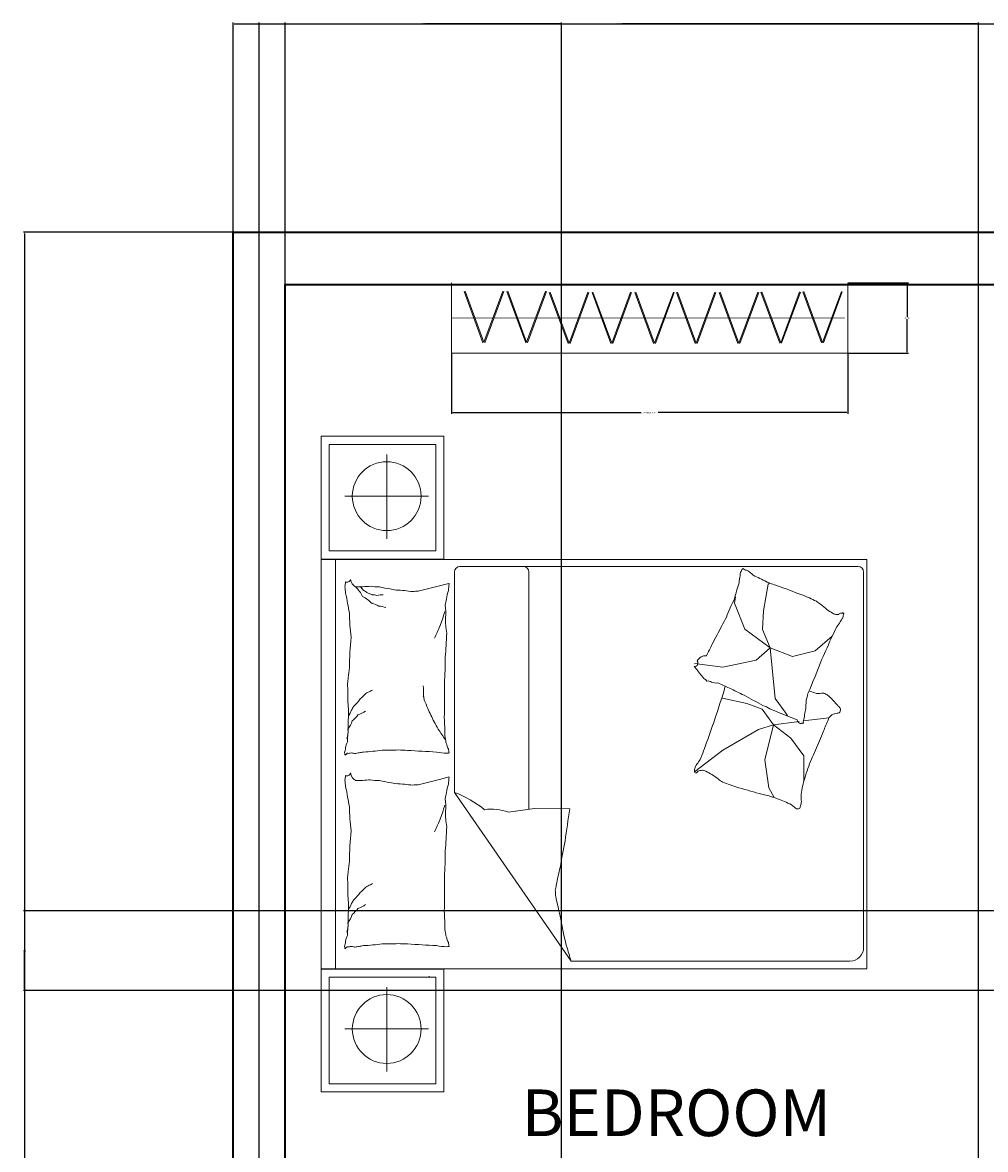
# Model space of a CAD drawing. Units: feet. Extents: x 1993 to 2298, y 2938 to 3641.
# Tile 9 of 11: x 1993 to 2141, y 3468 to 3641. Entities that reach past the tile are written whole.
import ezdxf

# ---------------------------------------------------------------- set-up
doc = ezdxf.new("R2010")
doc.units = ezdxf.units.FT
for name, color, linetype, lineweight in [('A-ANNO-DIMS', 2, 'Continuous', 18), ('A-AREA-IDEN', 7, 'Continuous', 18), ('furniture', 8, 'Continuous', 18), ('WAL', 7, 'Continuous', 35), ('wardrobe', 4, 'Continuous', 13)]:
    doc.layers.add(name, color=color, linetype=linetype, lineweight=lineweight)
doc.styles.add('DIM_FONT', font='SIMPLEX.shx', dxfattribs={"width": 0.8})
doc.styles.get("Standard").update_dxf_attribs({"font": 'arial.ttf'})
doc.dimstyles.get("Standard").update_dxf_attribs({"dimtxt": 0.18, "dimasz": 0.18, "dimexe": 0.18, "dimexo": 0.0625, "dimgap": 0.09, "dimtad": 0, "dimtih": 1, "dimtoh": 1, "dimdec": 4, "dimzin": 0, "dimdsep": 46, "dimtxsty": 'Standard', "dimcen": 0.09, "dimadec": 0, "dimazin": 0, "dimtfac": 1, "dimtdec": 4, "dimtofl": 0, "dimtmove": 0, "dimatfit": 3, "dimfxl": 1, "dimtolj": 1, "dimtzin": 0, "dimarcsym": 0})

# ---------------------------------------------------------------- blocks, each defined once
blk = doc.blocks.new('A$C79766A75')
for p, q in [((0.45, 1.9999), (0, 1.9999)), ((0, 1.9999), (0, 1.5499)), ((0.45, 1.5499), (0.45, 1.9999)), ((1.9506, 2), (0.4506, 2)), ((0.4506, 2), (0.4506, 0)), ((1.9506, 0), (1.9506, 2)), ((2.402, 1.9999), (1.952, 1.9999)), ((1.952, 1.9999), (1.952, 1.5499)), ((2.402, 1.5499), (2.402, 1.9999)), ((0.42, 1.9699), (0.03, 1.9699)), ((0.03, 1.9699), (0.03, 1.5799)), ((0.42, 1.5799), (0.42, 1.9699)), ((1.9506, 1.9476), (0.4506, 1.9476)), ((2.372, 1.9699), (1.982, 1.9699)), ((1.982, 1.9699), (1.982, 1.5799)), ((2.372, 1.5799), (2.372, 1.9699)), ((0.2304, 1.9125), (0.2304, 1.6061)), ((2.1824, 1.9125), (2.1824, 1.6061)), ((0.0743, 1.7595), (0.3834, 1.7595)), ((2.0263, 1.7595), (2.3354, 1.7595)), ((1.1461, 1.5617), (1.1254, 1.6443)), ((1.8553, 1.5617), (1.8346, 1.6443)), ((0.03, 1.5799), (0.42, 1.5799)), ((0.4234, 1.6034), (0.4228, 1.6034)), ((1.982, 1.5799), (2.372, 1.5799)), ((0, 1.5499), (0.45, 1.5499)), ((1.1536, 1.5317), (1.1461, 1.5617)), ((1.8628, 1.5317), (1.8553, 1.5617)), ((1.952, 1.5499), (2.402, 1.5499)), ((1.0972, 1.5115), (0.4791, 1.0841)), ((1.0972, 1.5115), (1.9048, 1.5115)), ((1.9248, 1.4915), (1.9248, 0.0322)), ((1.0383, 1.2184), (1.0246, 1.3138)), ((1.9048, 1.2389), (1.0354, 1.2389)), ((1.0365, 1.0883), (1.0383, 1.2184)), ((0.4791, 0.0622), (0.4791, 1.0841)), ((1.1731, 0.6316), (1.2523, 0.5276)), ((1.5696, 0.6317), (1.5559, 0.5286)), ((1.2523, 0.5276), (1.3274, 0.3973)), ((1.4223, 0.4407), (1.442, 0.5296)), ((1.5559, 0.5286), (1.5817, 0.4065)), ((1.6952, 0.4478), (1.7898, 0.4856)), ((1.7898, 0.4856), (1.8139, 0.4822)), ((1.4025, 0.3834), (1.4223, 0.4407)), ((1.6264, 0.355), (1.6952, 0.4478)), ((1.2167, 0.3736), (1.1139, 0.3597)), ((1.3452, 0.342), (1.2167, 0.3736)), ((1.3274, 0.3973), (1.3452, 0.342)), ((1.3452, 0.342), (1.4025, 0.3834)), ((1.5817, 0.4065), (1.6264, 0.355)), ((1.6264, 0.355), (1.6935, 0.3825)), ((1.6935, 0.3825), (1.7623, 0.379)), ((1.7623, 0.379), (1.8603, 0.3619)), ((1.1139, 0.3597), (1.0779, 0.3397)), ((1.2957, 0.2787), (1.3452, 0.342)), ((1.3452, 0.342), (1.3569, 0.2478)), ((1.4034, 0.3558), (1.3803, 0.2995)), ((1.4406, 0.3361), (1.3907, 0.3)), ((1.6264, 0.355), (1.4406, 0.3361)), ((1.5954, 0.2725), (1.6264, 0.355)), ((1.8603, 0.3619), (1.8636, 0.3554)), ((1.3803, 0.2995), (1.3626, 0.256)), ((1.3907, 0.3), (1.3787, 0.2914)), ((1.2305, 0.2313), (1.2957, 0.2787)), ((1.6161, 0.19), (1.5954, 0.2725)), ((1.1376, 0.2313), (1.2305, 0.2313)), ((1.3588, 0.2331), (1.3706, 0.1385)), ((1.6697, 0.1274), (1.6161, 0.19)), ((1.9048, 0.0122), (0.5291, 0.0122)), ((0.4506, 0), (1.9506, 0))]:
    blk.add_line(p, q)
for centre in [(0.2304, 1.7595), (2.1824, 1.7595)]:
    blk.add_circle(centre, 0.126)
for centre, radius, start, end in [((0.5232, 1.9139), 0.00342, 291.7883, 340.436), ((0.525, 1.9085), 0.00232, 340.436, 101.8931), ((0.5246, 1.9378), 0.0251, 274.3025, 291.7883), ((0.5311, 1.9093), 0.00428, 201.9904, 281.8931), ((0.5465, 1.8994), 0.0156, 158.579, 201.9904), ((0.5486, 1.9393), 0.0289, 239.3487, 274.3025), ((0.5458, 1.8568), 0.0539, 59.3487, 84.7408), ((0.546, 1.0829), 0.8208, 84.7408, 88.0921), ((0.6118, 2.0005), 0.0992, 254.0648, 274.2159), ((0.6775, 1.9817), 0.0992, 233.9136, 254.0648), ((0.6362, 0.406), 1.4943, 88.0921, 90.5757), ((0.7737, 2.1075), 0.234, 242.7604, 249.1397), ((0.7591, 1.0293), 0.8732, 90.5757, 94.8018), ((0.7631, 2.1919), 0.2897, 267.4614, 274.8018), ((0.8143, 2.0532), 0.1524, 259.8101, 267.4614), ((0.7515, 1.3747), 0.5293, 79.8101, 83.9133), ((1.1117, 1.6625), 0.2422, 97.5469, 105.744), ((1.0352, 2.2041), 0.3048, 278.4372, 285.744), ((1.1179, 2.0719), 0.1611, 270, 278.4372), ((1.1592, 2.0011), 0.0904, 258.7276, 270), ((1.1709, 1.9049), 0.0131, 153.4195, 258.7276), ((1.2325, 1.9139), 0.00342, 291.7883, 340.436), ((1.2342, 1.9085), 0.00232, 340.436, 101.8931), ((1.2338, 1.9378), 0.0251, 274.3025, 291.7883), ((1.2404, 1.9093), 0.00428, 201.9904, 281.8931), ((1.2558, 1.8994), 0.0156, 158.579, 201.9904), ((1.2578, 1.9393), 0.0289, 239.3487, 274.3025), ((1.2551, 1.8568), 0.0539, 59.3487, 84.7408), ((1.2552, 1.0829), 0.8208, 84.7408, 88.0921), ((1.3211, 2.0005), 0.0992, 254.0648, 274.2159), ((1.3868, 1.9817), 0.0992, 233.9136, 254.0648), ((1.3455, 0.406), 1.4943, 88.0921, 90.5757), ((1.4829, 2.1075), 0.234, 242.7604, 249.1397), ((1.4683, 1.0293), 0.8732, 90.5757, 94.8018), ((1.4724, 2.1919), 0.2897, 267.4614, 274.8018), ((1.5236, 2.0532), 0.1524, 259.8101, 267.4614), ((1.4607, 1.3747), 0.5293, 79.8101, 83.9133), ((1.821, 1.6625), 0.2422, 97.5469, 105.744), ((1.7444, 2.2041), 0.3048, 278.4372, 285.744), ((1.8271, 2.0719), 0.1611, 270, 278.4372), ((1.8684, 2.0011), 0.0904, 258.7276, 270), ((1.8802, 1.9049), 0.0131, 153.4195, 258.7276), ((0.4996, 1.8889), 0.0328, 338.579, 8.1335), ((0.2896, 1.8253), 0.246, 8.1335, 12.1095), ((0.7297, 1.8867), 0.1983, 187.6809, 192.1095), ((0.7304, 1.9449), 0.0992, 216.1766, 233.9136), ((0.7661, 1.8961), 0.0992, 198.4397, 216.1766), ((0.738, 1.949), 0.0768, 231.6114, 242.7604), ((0.974, 2.1633), 0.3916, 226.1885, 231.6114), ((0.8451, 0.8466), 1.049, 83.9133, 90), ((1.046, 1.2129), 0.6827, 90, 97.5469), ((1.171, 1.8579), 0.0342, 94.4002, 153.4195), ((1.6324, 1.8735), 0.4918, 180, 186.2324), ((1.2088, 1.8889), 0.0328, 338.579, 8.1335), ((0.9988, 1.8253), 0.246, 8.1335, 12.1095), ((1.4389, 1.8867), 0.1983, 187.6809, 192.1095), ((1.4396, 1.9449), 0.0992, 216.1766, 233.9136), ((1.4753, 1.8961), 0.0992, 198.4397, 216.1766), ((1.4473, 1.949), 0.0768, 231.6114, 242.7604), ((1.6833, 2.1633), 0.3916, 226.1885, 231.6114), ((1.5543, 0.8466), 1.049, 83.9133, 90), ((1.7552, 1.2129), 0.6827, 90, 97.5469), ((1.7511, 1.9723), 0.1399, 297.2036, 314.9024), ((1.8802, 1.8579), 0.0342, 94.4002, 153.4195), ((2.3416, 1.8735), 0.4918, 180, 186.2324), ((1.4472, 1.8987), 0.9131, 183.3687, 187.6809), ((0.9057, 1.9982), 0.2252, 219.0349, 226.1885), ((0.7932, 1.8591), 0.0493, 208.3168, 219.0349), ((0.9392, 1.9062), 0.2002, 203.0028, 208.3168), ((1.3446, 1.7858), 0.204, 170.3156, 180), ((2.1565, 1.8987), 0.9131, 183.3687, 187.6809), ((1.615, 1.9982), 0.2252, 219.0349, 226.1885), ((1.5025, 1.8591), 0.0493, 208.3168, 219.0349), ((1.6484, 1.9062), 0.2002, 203.0028, 208.3168), ((1.6908, 1.9123), 0.1399, 314.9024, 332.6012), ((1.6307, 1.8895), 0.2056, 338.1851, 341.2201), ((1.6887, 1.8881), 0.1511, 334.6449, 338.1851), ((1.7896, 1.8667), 0.0526, 318.5571, 334.6449), ((1.784, 1.9167), 0.0899, 306.2641, 318.5571), ((2.0538, 1.7858), 0.204, 170.3156, 180), ((1.2208, 1.7573), 0.6787, 178.3669, 183.3687), ((2.0027, 1.5994), 0.882, 167.8016, 170.3156), ((1.9301, 1.7573), 0.6787, 178.3669, 183.3687), ((1.6404, 1.8023), 0.1399, 343.485, 354.3689), ((1.6554, 1.8529), 0.1399, 332.6012, 343.485), ((1.7653, 1.8132), 0.0562, 341.2201, 0), ((1.73, 1.7719), 0.0915, 0, 14.6851), ((2.7119, 1.5994), 0.882, 167.8016, 170.3156), ((0.8192, 1.792), 0.3171, 347.8016, 351.9949), ((1.5284, 1.792), 0.3171, 347.8016, 351.9949), ((1.9066, 1.6447), 1.3652, 176.945, 178.3669), ((0.4711, 1.7556), 0.6588, 351.9949, 357.3351), ((2.6158, 1.6447), 1.3652, 176.945, 178.3669), ((1.1803, 1.7556), 0.6588, 351.9949, 357.3351), ((14.1519, 0.85), 13.6356, 176.49514, 176.94504), ((1.0578, 1.6474), 0.0677, 357.3351, 14.0452), ((14.8612, 0.85), 13.6356, 176.49514, 176.94504), ((1.767, 1.6474), 0.0677, 357.3351, 14.0452), ((1.226, 2.0834), 0.5066, 290.6743, 294.3265), ((1.4305, 1.6796), 0.058, 274.0828, 290.6743), ((1.4679, 1.8969), 0.2721, 266.4448, 274.0828), ((0.8521, 1.5209), 0.3212, 170.0016, 176.4951), ((0.6583, 0.9067), 0.7387, 64.6889, 66.5156), ((0.7015, 0.888), 0.7387, 66.5156, 68.3423), ((1.5613, 1.5209), 0.3212, 170.0016, 176.4951), ((0.9025, 2.1618), 0.7286, 302.135, 305.8263), ((1.1895, 1.8508), 0.3126, 296.4985, 302.135), ((0.7658, 2.8912), 1.4323, 294.3265, 296.4985), ((1.3675, 0.9067), 0.7387, 64.6889, 66.5156), ((1.4107, 0.888), 0.7387, 66.5156, 68.3423), ((0.513, 1.535), 0.0193, 350.0016, 16.6978), ((0.5322, 1.5304), 0.00132, 16.6978, 97.1204), ((0.5579, 1.4467), 0.0875, 97.1204, 106.2212), ((0.5822, 1.4654), 0.0767, 106.2212, 117.2841), ((0.5507, 1.5832), 0.0453, 282.869, 297.2841), ((0.5623, 1.6885), 0.1459, 273.574, 282.869), ((0.589, 2.7103), 1.164, 270.2865, 273.574), ((0.7584, 7.2662), 5.7185, 269.0296, 270.2865), ((0.9401, 4.9065), 3.3622, 267.3904, 269.0296), ((0.9811, 2.7573), 1.2165, 265.3824, 267.3904), ((0.8583, 0.139), 1.4048, 85.3824, 87.2509), ((1.0175, 1.3138), 0.2301, 87.2509, 101.5586), ((0.7501, 0.8688), 0.7387, 68.3423, 70.572), ((0.8043, 0.8497), 0.7387, 70.572, 72.8018), ((1.0449, 1.6886), 0.1459, 263.5659, 281.5586), ((1.1099, 1.6599), 0.1197, 252.6136, 263.5659), ((1.0587, 1.3144), 0.2297, 72.6136, 80.5159), ((1.108, 1.2635), 0.2708, 80.5159, 85.9171), ((1.1535, 1.5308), 0.000917, 85.9171, 194.0449), ((1.2222, 1.535), 0.0193, 350.0016, 16.6978), ((1.2414, 1.5304), 0.00132, 16.6978, 97.1204), ((1.2671, 1.4467), 0.0875, 97.1204, 106.2212), ((1.2914, 1.4654), 0.0767, 106.2212, 117.2841), ((1.2599, 1.5832), 0.0453, 282.869, 297.2841), ((1.2716, 1.6885), 0.1459, 273.574, 282.869), ((1.2982, 2.7103), 1.164, 270.2865, 273.574), ((1.4677, 7.2662), 5.7185, 269.0296, 270.2865), ((1.6493, 4.9065), 3.3622, 267.3904, 269.0296), ((1.6903, 2.7573), 1.2165, 265.3824, 267.3904), ((1.5676, 0.139), 1.4048, 85.3824, 87.2509), ((1.7268, 1.3138), 0.2301, 87.2509, 101.5586), ((1.4594, 0.8688), 0.7387, 68.3423, 70.572), ((1.5136, 0.8497), 0.7387, 70.572, 72.8018), ((1.7541, 1.6886), 0.1459, 263.5659, 281.5586), ((1.8192, 1.6599), 0.1197, 252.6136, 263.5659), ((1.7679, 1.3144), 0.2297, 72.6136, 80.5159), ((1.8172, 1.2635), 0.2708, 80.5159, 85.9171), ((1.8627, 1.5308), 0.000917, 85.9171, 194.0449), ((0.745, 1.6407), 0.3751, 320.3555, 339.8512), ((1.9048, 1.4915), 0.02, 0, 90), ((0.8556, 1.3759), 0.1801, 339.8512, 8.1356), ((1.9048, 1.2589), 0.02, 270, 0), ((-0.1888, 5.1029), 4.0646, 280.7276, 282.9255), ((0.7282, 1.1989), 0.0581, 262.2696, 280.7276), ((0.7833, 1.3309), 0.1942, 256.8096, 262.2696), ((0.2481, -1.3253), 2.5158, 76.8096, 78.3259), ((0.3953, -1.4284), 2.588, 78.3259, 80.505), ((-0.0248, 2.8487), 1.8351, 285.9352, 287.7364), ((0.3872, 1.7415), 0.6574, 282.9255, 285.9352), ((0.413, -2.64), 3.7801, 80.505, 82.308), ((1.1752, 0.6267), 0.0063, 166.7192, 233.4208), ((1.1734, 0.6272), 0.00443, 93.9484, 166.7192), ((1.163, 0.6103), 0.0142, 10.4074, 53.4208), ((1.1755, 0.5964), 0.0352, 69.6548, 93.9484), ((1.1669, 0.5731), 0.0601, 51.4146, 69.6548), ((1.2538, 0.682), 0.0792, 231.4146, 247.2931), ((1.1426, 1.1456), 0.6605, 306.2163, 307.2151), ((1.7751, 0.3162), 0.3825, 126.2163, 127.5287), ((1.5806, 0.5924), 0.0452, 127.5287, 134.1274), ((1.5093, 0.6825), 0.0697, 308.8136, 314.1274), ((1.5706, 0.6318), 0.0127, 176.7545, 308.8136), ((1.5621, 0.59), 0.0359, 356.7545, 62.7098), ((0.8605, 0.749), 0.352, 329.0944, 333.1821), ((1.1396, 0.6079), 0.0393, 333.1821, 345.4291), ((1.1011, 0.5989), 0.0771, 2.7286, 10.4074), ((1.1628, 0.6019), 0.0153, 345.4291, 2.7286), ((1.5463, 1.3811), 0.8371, 247.2931, 249.8713), ((3.0113, 5.3783), 5.0942, 249.8713, 250.9164), ((1.4828, 0.5833), 0.0226, 324.1064, 8.0492), ((1.4519, 0.6426), 0.0774, 313.5224, 324.1064), ((1.383, 0.7705), 0.2176, 307.2151, 313.5224), ((0.2201, -2.1858), 3.0972, 62.7098, 63.5853), ((1.2077, 0.4922), 0.081, 140.2995, 153.9265), ((0.9961, 0.6678), 0.194, 320.2995, 329.0944), ((2.374, 3.5362), 3.145, 250.9164, 253.3915), ((2.4089, 0.1204), 1.0054, 154.9471, 157.5838), ((1.5435, 0.5526), 0.0458, 157.5838, 188.0492), ((2.5711, 2.3551), 2.0162, 242.5001, 243.5853), ((4.5245, 5.9445), 6.1019, 242.15178, 242.50014), ((3.0311, -0.112), 2.003, 162.1604, 164.7375), ((1.3115, 0.4414), 0.1965, 153.9265, 162.1604), ((2.9813, -0.2643), 1.6868, 152.9116, 154.9471), ((1.5084, 0.6341), 0.1166, 253.3915, 259.2634), ((-0.9881, -4.647), 5.8383, 62.15178, 62.50792), ((1.5182, -0.068), 0.6236, 62.5079, 69.2514), ((1.7121, 0.0657), 0.43, 69.2514, 77.3748), ((1.8682, 0.4049), 0.063, 77.3748, 93.3881), ((1.8955, 0.5247), 0.0599, 256.9598, 273.3881), ((1.9257, 0.5082), 0.0509, 238.3083, 256.9598), ((1.9201, 0.4587), 0.0058, 180.9614, 238.3083), ((2.6887, -0.0186), 1.6481, 164.7375, 166.159), ((2.8096, -0.3311), 1.5652, 150.064, 152.9116), ((-0.5166, 1.5491), 2.6619, 333.6668, 334.8268), ((1.8435, 0.4743), 0.0755, 310.5086, 333.6668), ((1.9279, 0.441), 0.0168, 130.5086, 180.9614), ((0.5589, 0.5062), 0.5454, 343.6878, 346.159), ((1.2176, 0.4627), 0.2143, 330.064, 337.7645), ((-1.4109, 1.284), 2.6619, 338.0627, 339.2227), ((0.9098, 0.4035), 0.1798, 339.2227, 343.6878), ((3.4079, -0.2212), 1.6481, 160.3416, 161.7631), ((1.3456, 0.5261), 0.5454, 339.2919, 341.7631), ((1.701, 0.4319), 0.1798, 334.8268, 339.2919), ((0.9882, 0.3177), 0.0755, 314.9045, 338.0627), ((3.6966, -0.4634), 2.003, 157.7645, 160.3416), ((1.0533, 0.2524), 0.0168, 134.9045, 185.3572), ((1.0424, 0.2513), 0.0058, 185.3572, 242.7041), ((1.3694, 0.234), 0.0231, 107.1867, 157.7645), ((1.0631, 0.2914), 0.0509, 242.7041, 261.3557), ((1.0645, 0.3003), 0.0599, 261.3557, 277.784), ((1.0811, 0.1786), 0.063, 81.7707, 97.784), ((1.0286, -0.1846), 0.43, 73.6473, 81.7707), ((0.974, -0.3705), 0.6236, 66.9038, 73.6473), ((1.3465, 0.2383), 0.00467, 287.1867, 70.6201), ((1.3486, 0.2247), 0.0092, 70.6201, 94.2593), ((1.3563, 0.267), 0.034, 262.0178, 274.2593), ((1.4091, 0.4221), 0.1955, 255.1193, 262.0178), ((1.358, 0.0507), 0.1794, 75.1193, 82.3216), ((1.4096, 0.153), 0.0712, 82.3216, 94.5118), ((1.4285, 0.2893), 0.0663, 261.8784, 274.5118), ((1.4755, 0.332), 0.1166, 248.9957, 261.8784), ((2.7121, 3.1012), 3.145, 246.5205, 248.9957), ((2.4175, -0.1202), 1.0054, 160.6552, 161.9797), ((1.9797, 0.1108), 0.1965, 149.5306, 157.7645), ((-1.0716, -5.1672), 5.8383, 66.54766, 66.9038), ((3.6805, 5.7866), 6.1019, 246.54766, 246.89602), ((2.0773, 2.0287), 2.0162, 246.896, 247.9812), ((1.4382, 0.1619), 0.0226, 328.5023, 12.4451), ((1.505, 0.1766), 0.0458, 161.9797, 192.4451), ((3.6993, 4.7998), 5.0942, 245.4754, 246.5205), ((1.6279, 0.2819), 0.194, 315.9036, 324.6985), ((1.856, 0.1288), 0.081, 135.9036, 149.5306), ((0.1602, -2.7118), 3.0972, 67.1056, 67.9812), ((1.3512, 0.1084), 0.0359, 1.1504, 67.1056), ((1.2874, 0.2845), 0.2176, 311.611, 317.9183), ((1.3914, 0.1905), 0.0774, 317.9183, 328.5023), ((2.051, 0.8725), 0.8371, 242.8972, 245.4754), ((1.7162, 0.1388), 0.0393, 328.7862, 341.0332), ((1.4661, 0.3294), 0.352, 324.6985, 328.7862), ((1.3997, 0.1094), 0.0127, 181.1504, 313.2095), ((1.3607, 0.1509), 0.0697, 313.2095, 318.5233), ((1.4468, 0.0748), 0.0452, 131.9246, 138.5233), ((1.6722, -0.1762), 0.3825, 130.6122, 131.9246), ((0.9933, 0.6156), 0.6605, 310.6122, 311.611), ((1.7576, 0.1689), 0.0792, 227.0187, 242.8972), ((1.6963, 0.0438), 0.0601, 47.0187, 65.2589), ((1.737, 0.0526), 0.0352, 65.2589, 89.5525), ((1.7345, 0.1188), 0.0153, 341.0332, 358.3327), ((1.6723, 0.1058), 0.0771, 358.3327, 6.0115), ((1.7401, 0.0928), 0.0142, 6.0115, 49.0249), ((1.756, 0.0832), 0.00443, 89.5525, 162.3233), ((1.7602, 0.0924), 0.0063, 162.3233, 229.0249), ((0.5291, 0.0622), 0.05, 180, 270), ((1.9048, 0.0322), 0.02, 270, 0)]:
    blk.add_arc(centre, radius, start, end)
at = {"style": 'DIM_FONT', "text_generation_flag": 4, "width": 0.8, "flags": 9}
for tag in ['XSIZE', 'YSIZE']:
    blk.add_attdef(tag, (1.9506, 2), '', height=0.0005, rotation=180, dxfattribs=at)
blk = doc.blocks.new('WARDROBE-PLAN')
for p, q in [((4.82, 1.61), (1.93, 9.47)), ((4.96, 1.67), (2.08, 9.52)), ((4.96, 1.67), (7.85, 9.52)), ((5.11, 1.61), (7.99, 9.46)), ((11.37, 1.61), (8.49, 9.46)), ((11.51, 1.67), (8.63, 9.52)), ((11.51, 1.67), (14.4, 9.52)), ((11.66, 1.61), (14.54, 9.46)), ((17.87, 1.47), (14.98, 9.32)), ((18.01, 1.52), (15.13, 9.37)), ((18.01, 1.52), (20.9, 9.37)), ((18.16, 1.47), (21.04, 9.32)), ((24.42, 1.47), (21.53, 9.32)), ((24.56, 1.52), (21.68, 9.37)), ((24.56, 1.52), (27.45, 9.37)), ((24.71, 1.47), (27.59, 9.32)), ((30.97, 1.47), (28.09, 9.32)), ((31.11, 1.52), (28.23, 9.37)), ((31.11, 1.52), (34, 9.37)), ((31.26, 1.47), (34.14, 9.32)), ((37.35, 1.47), (34.47, 9.32)), ((37.5, 1.52), (34.62, 9.37)), ((37.5, 1.52), (40.38, 9.37)), ((37.64, 1.47), (40.53, 9.32)), ((43.9, 1.46), (41.02, 9.32)), ((44.05, 1.52), (41.17, 9.37)), ((44.05, 1.52), (46.93, 9.37)), ((44.19, 1.46), (47.08, 9.32)), ((50.31, 1.52), (47.43, 9.37)), ((50.46, 1.57), (47.57, 9.42)), ((50.46, 1.57), (53.34, 9.42)), ((50.6, 1.52), (53.49, 9.37)), ((56.72, 1.57), (53.83, 9.42)), ((56.86, 1.62), (53.98, 9.47)), ((56.86, 1.62), (59.75, 9.47)), ((57.01, 1.57), (59.89, 9.42)), ((0, 5.4), (60.23, 5.39))]:
    blk.add_line(p, q)
blk.add_lwpolyline([(0, 10.78), (0, 0.01), (60.75, 0), (60.75, 10.78)])
blk = doc.blocks.new('*D36')
at = {"layer": 'A-ANNO-DIMS', "color": 0, "lineweight": -2, "transparency": 16777216}
for p, q in [((2059.25, 3589.94), (2059.25, 3580.71)), ((2120, 3589.94), (2120, 3580.71)), ((2059.43, 3580.89), (2088.32, 3580.89)), ((2119.82, 3580.89), (2090.93, 3580.89))]:
    blk.add_line(p, q, dxfattribs=at)
at = {"layer": 'A-ANNO-DIMS', "color": 0, "transparency": 16777216}
for points in [[(2059.43, 3580.92), (2059.43, 3580.86), (2059.25, 3580.89)], [(2119.82, 3580.92), (2119.82, 3580.86), (2120, 3580.89)]]:
    blk.add_solid(points, dxfattribs=at)
at = {"layer": 'Defpoints', "color": 0, "transparency": 16777216}
for p in [(2059.25, 3590), (2120, 3590), (2120, 3580.89)]:
    blk.add_point(p, dxfattribs=at)
at = {"layer": 'A-ANNO-DIMS', "color": 0, "transparency": 16777216, "insert": (2089.62, 3580.89), "char_height": 0.18, "attachment_point": 5}
blk.add_mtext('\\A1;WARDROBE 61 TYP.', dxfattribs=at)
blk = doc.blocks.new('*D37')
at = {"layer": 'A-ANNO-DIMS', "color": 0, "lineweight": -2, "transparency": 16777216}
for p, q in [((2120.06, 3600.78), (2129.29, 3600.78)), ((2129.11, 3600.6), (2129.11, 3595.57)), ((2129.11, 3590.18), (2129.11, 3595.21)), ((2120.06, 3590), (2129.29, 3590))]:
    blk.add_line(p, q, dxfattribs=at)
at = {"layer": 'A-ANNO-DIMS', "color": 0, "transparency": 16777216}
for points in [[(2129.08, 3600.6), (2129.14, 3600.6), (2129.11, 3600.78)], [(2129.08, 3590.18), (2129.14, 3590.18), (2129.11, 3590)]]:
    blk.add_solid(points, dxfattribs=at)
at = {"layer": 'Defpoints', "color": 0, "transparency": 16777216}
for p in [(2120, 3600.78), (2129.11, 3600.78), (2120, 3590)]:
    blk.add_point(p, dxfattribs=at)
at = {"layer": 'A-ANNO-DIMS', "color": 0, "transparency": 16777216, "insert": (2129.11, 3595.39), "char_height": 0.18, "attachment_point": 5}
blk.add_mtext('\\A1;11 TYP.', dxfattribs=at)
blk = doc.blocks.new('*D54')
at = {"layer": 'A-ANNO-DIMS', "color": 0, "lineweight": -2, "transparency": 16777216}
for p, q in [((2025.76, 3608.6), (2025.76, 3640.68)), ((2025.94, 3640.5), (2145.47, 3640.5)), ((2265.58, 3640.5), (2146.05, 3640.5)), ((2265.76, 3608.6), (2265.76, 3640.68))]:
    blk.add_line(p, q, dxfattribs=at)
at = {"layer": 'A-ANNO-DIMS', "color": 0, "transparency": 16777216}
for points in [[(2025.94, 3640.53), (2025.94, 3640.47), (2025.76, 3640.5)], [(2265.58, 3640.53), (2265.58, 3640.47), (2265.76, 3640.5)]]:
    blk.add_solid(points, dxfattribs=at)
at = {"layer": 'Defpoints', "color": 0, "transparency": 16777216}
for p in [(2265.76, 3640.5), (2025.76, 3608.53), (2265.76, 3608.53)]:
    blk.add_point(p, dxfattribs=at)
at = {"layer": 'A-ANNO-DIMS', "color": 0, "transparency": 16777216, "insert": (2145.76, 3640.5), "char_height": 0.18, "attachment_point": 5}
blk.add_mtext('\\A1;240', dxfattribs=at)
blk = doc.blocks.new('*D56')
at = {"layer": 'A-ANNO-DIMS', "color": 0, "lineweight": -2, "transparency": 16777216}
for p, q in [((2025.7, 3608.53), (1993.61, 3608.53)), ((1993.79, 3608.35), (1993.79, 3289.45)), ((1993.79, 2970.18), (1993.79, 3289.08)), ((2029.7, 2970), (1993.61, 2970))]:
    blk.add_line(p, q, dxfattribs=at)
at = {"layer": 'A-ANNO-DIMS', "color": 0, "transparency": 16777216}
for points in [[(1993.76, 3608.35), (1993.82, 3608.35), (1993.79, 3608.53)], [(1993.76, 2970.18), (1993.82, 2970.18), (1993.79, 2970)]]:
    blk.add_solid(points, dxfattribs=at)
at = {"layer": 'Defpoints', "color": 0, "transparency": 16777216}
for p in [(1993.79, 3608.53), (2025.76, 3608.53), (2029.76, 2970)]:
    blk.add_point(p, dxfattribs=at)
at = {"layer": 'A-ANNO-DIMS', "color": 0, "transparency": 16777216, "insert": (1993.79, 3289.27), "char_height": 0.18, "attachment_point": 5}
blk.add_mtext('\\A1;638.5', dxfattribs=at)
blk = doc.blocks.new('*D59')
at = {"layer": 'A-ANNO-DIMS', "color": 0, "lineweight": -2, "transparency": 16777216}
for p, q in [((2140, 3048.6), (2140, 3640.68)), ((2140.18, 3640.5), (2144.79, 3640.5)), ((2149.82, 3640.5), (2145.21, 3640.5)), ((2150, 3048.6), (2150, 3640.68))]:
    blk.add_line(p, q, dxfattribs=at)
at = {"layer": 'A-ANNO-DIMS', "color": 0, "transparency": 16777216}
for points in [[(2140.18, 3640.53), (2140.18, 3640.47), (2140, 3640.5)], [(2149.82, 3640.53), (2149.82, 3640.47), (2150, 3640.5)]]:
    blk.add_solid(points, dxfattribs=at)
at = {"layer": 'Defpoints', "color": 0, "transparency": 16777216}
for p in [(2150, 3640.5), (2140, 3048.53), (2150, 3048.53)]:
    blk.add_point(p, dxfattribs=at)
at = {"layer": 'A-ANNO-DIMS', "color": 0, "transparency": 16777216, "insert": (2145, 3640.5), "char_height": 0.18, "attachment_point": 5}
blk.add_mtext('\\A1;10', dxfattribs=at)
blk = doc.blocks.new('*D70')
at = {"layer": 'A-ANNO-DIMS', "color": 0, "lineweight": -2, "transparency": 16777216}
for p, q in [((2149.7, 3504.53), (1993.61, 3504.53)), ((1993.79, 3504.35), (1993.79, 3498.61)), ((1993.79, 3492.51), (1993.79, 3498.25)), ((2149.7, 3492.33), (1993.61, 3492.33))]:
    blk.add_line(p, q, dxfattribs=at)
at = {"layer": 'A-ANNO-DIMS', "color": 0, "transparency": 16777216}
for points in [[(1993.76, 3504.35), (1993.82, 3504.35), (1993.79, 3504.53)], [(1993.76, 3492.51), (1993.82, 3492.51), (1993.79, 3492.33)]]:
    blk.add_solid(points, dxfattribs=at)
at = {"layer": 'Defpoints', "color": 0, "transparency": 16777216}
for p in [(1993.79, 3504.53), (2149.76, 3504.53), (2149.76, 3492.33)]:
    blk.add_point(p, dxfattribs=at)
at = {"layer": 'A-ANNO-DIMS', "color": 0, "transparency": 16777216, "insert": (1993.79, 3498.43), "char_height": 0.18, "attachment_point": 5}
blk.add_mtext('\\A1;12.2', dxfattribs=at)
blk = doc.blocks.new('*D75')
at = {"layer": 'A-ANNO-DIMS', "color": 0, "lineweight": -2, "transparency": 16777216}
for p, q in [((2029.76, 3008.6), (2029.76, 3640.68)), ((2029.94, 3640.5), (2084.42, 3640.5)), ((2139.82, 3640.5), (2085.33, 3640.5)), ((2140, 3008.6), (2140, 3640.68))]:
    blk.add_line(p, q, dxfattribs=at)
at = {"layer": 'A-ANNO-DIMS', "color": 0, "transparency": 16777216}
for points in [[(2029.94, 3640.53), (2029.94, 3640.47), (2029.76, 3640.5)], [(2139.82, 3640.53), (2139.82, 3640.47), (2140, 3640.5)]]:
    blk.add_solid(points, dxfattribs=at)
at = {"layer": 'Defpoints', "color": 0, "transparency": 16777216}
for p in [(2140, 3640.5), (2029.76, 3008.53), (2140, 3008.53)]:
    blk.add_point(p, dxfattribs=at)
at = {"layer": 'A-ANNO-DIMS', "color": 0, "transparency": 16777216, "insert": (2084.88, 3640.5), "char_height": 0.18, "attachment_point": 5}
blk.add_mtext('\\A1;110.24', dxfattribs=at)
blk = doc.blocks.new('*D76')
at = {"layer": 'A-ANNO-DIMS', "color": 0, "lineweight": -2, "transparency": 16777216}
for p, q in [((2033.76, 3188.6), (2033.76, 3640.68)), ((2033.94, 3640.5), (2054.54, 3640.5)), ((2075.93, 3640.5), (2055.33, 3640.5)), ((2076.11, 3188.6), (2076.11, 3640.68))]:
    blk.add_line(p, q, dxfattribs=at)
at = {"layer": 'A-ANNO-DIMS', "color": 0, "transparency": 16777216}
for points in [[(2033.94, 3640.53), (2033.94, 3640.47), (2033.76, 3640.5)], [(2075.93, 3640.53), (2075.93, 3640.47), (2076.11, 3640.5)]]:
    blk.add_solid(points, dxfattribs=at)
at = {"layer": 'Defpoints', "color": 0, "transparency": 16777216}
for p in [(2076.11, 3640.5), (2033.76, 3188.53), (2076.11, 3188.53)]:
    blk.add_point(p, dxfattribs=at)
at = {"layer": 'A-ANNO-DIMS', "color": 0, "transparency": 16777216, "insert": (2054.93, 3640.5), "char_height": 0.18, "attachment_point": 5}
blk.add_mtext('\\A1;42.35', dxfattribs=at)

msp = doc.modelspace()

# ---------------------------------------------------------------- linework, layer by layer
at = {"layer": 'WAL'}
for p, q in [((2025.7583, 3608.5338), (2265.7583, 3608.5338)), ((2025.7583, 3008.5338), (2025.7583, 3608.5338)), ((2033.7583, 3184.5338), (2033.7583, 3600.5338)), ((2033.7583, 3600.5338), (2145.7583, 3600.5338))]:
    msp.add_line(p, q, dxfattribs=at)

# ---------------------------------------------------------------- block references
at = {"layer": 'furniture', "xscale": 41.83725109546206, "yscale": 41.83725109546206, "zscale": 41.83725109546206, "rotation": 90}
msp.add_blockref('A$C79766A75', (2122.9212, 3476.78), dxfattribs=at)
at = {"layer": 'wardrobe'}
msp.add_blockref('WARDROBE-PLAN', (2059.247, 3590), dxfattribs=at)

# ---------------------------------------------------------------- texts
at = {"layer": 'A-AREA-IDEN'}
msp.add_text('BEDROOM', height=7.14808, dxfattribs=at).set_placement((2070, 3470))

# ---------------------------------------------------------------- dimensions: what is measured, and where the dimension line sits
at = {"layer": 'A-ANNO-DIMS'}
for base, p1, p2, override, picture, middle in [((2265.7583, 3640.4988), (2025.7583, 3608.5338), (2265.7583, 3608.5338), {"dimdec": 0, "dimlfac": 1, "dimrnd": 0, "dimzin": 0, "dimdsep": 46, "dimlunit": 2}, '*D54', (2145.7583, 3640.4988)), ((2140, 3640.4988), (2029.7583, 3008.5338), (2140, 3008.5338), {"dimdec": 2, "dimlfac": 1, "dimrnd": 0, "dimzin": 0, "dimdsep": 46, "dimlunit": 2}, '*D75', (2084.8792, 3640.4988)), ((2076.1089, 3640.4988), (2033.7583, 3188.5338), (2076.1089, 3188.5338), {"dimdec": 2, "dimlfac": 1, "dimrnd": 0, "dimzin": 0, "dimdsep": 46, "dimlunit": 2}, '*D76', (2054.9336, 3640.4988)), ((2150, 3640.4988), (2140, 3048.5338), (2150, 3048.5338), {"dimdec": 0, "dimlfac": 1, "dimrnd": 0, "dimzin": 0, "dimdsep": 46, "dimlunit": 2}, '*D59', (2145, 3640.4988))]:
    dim = msp.add_linear_dim(base=base, p1=p1, p2=p2, dimstyle='Standard', override=override, dxfattribs=at)
    dim.commit()
    dim.dimension.update_dxf_attribs({"geometry": picture, "text_midpoint": middle})
for base, p1, p2, picture, middle in [((1993.7933, 3608.5338), (2029.7583, 2970), (2025.7583, 3608.5338), '*D56', (1993.7933, 3289.2669)), ((1993.7933, 3504.5338), (2149.7583, 3492.3338), (2149.7583, 3504.5338), '*D70', (1993.7933, 3498.4338))]:
    dim = msp.add_linear_dim(base=base, p1=p1, p2=p2, angle=90, dimstyle='Standard', override={"dimdec": 1, "dimlfac": 1, "dimrnd": 0, "dimzin": 0, "dimdsep": 46, "dimlunit": 2}, dxfattribs=at)
    dim.commit()
    dim.dimension.update_dxf_attribs({"geometry": picture, "text_midpoint": middle})
dim = msp.add_linear_dim(base=(2129.1148, 3600.7834), p1=(2120.0015, 3590), p2=(2120.0015, 3600.7834), angle=90, text='<> TYP.', dimstyle='Standard', override={"dimdec": 0, "dimlfac": 1, "dimrnd": 0, "dimzin": 0, "dimdsep": 46, "dimlunit": 2}, dxfattribs=at)
dim.commit()
dim.dimension.update_dxf_attribs({"geometry": '*D37', "text_midpoint": (2129.1148, 3595.3917)})
dim = msp.add_linear_dim(base=(2120.0015, 3580.8868), p1=(2059.2467, 3590), p2=(2120.0015, 3590), text='WARDROBE <> TYP.', dimstyle='Standard', override={"dimdec": 0, "dimlfac": 1, "dimrnd": 0, "dimzin": 0, "dimdsep": 46, "dimlunit": 2}, dxfattribs=at)
dim.commit()
dim.dimension.update_dxf_attribs({"geometry": '*D36', "text_midpoint": (2089.6241, 3580.8868)})

doc.saveas('drawing.dxf')
